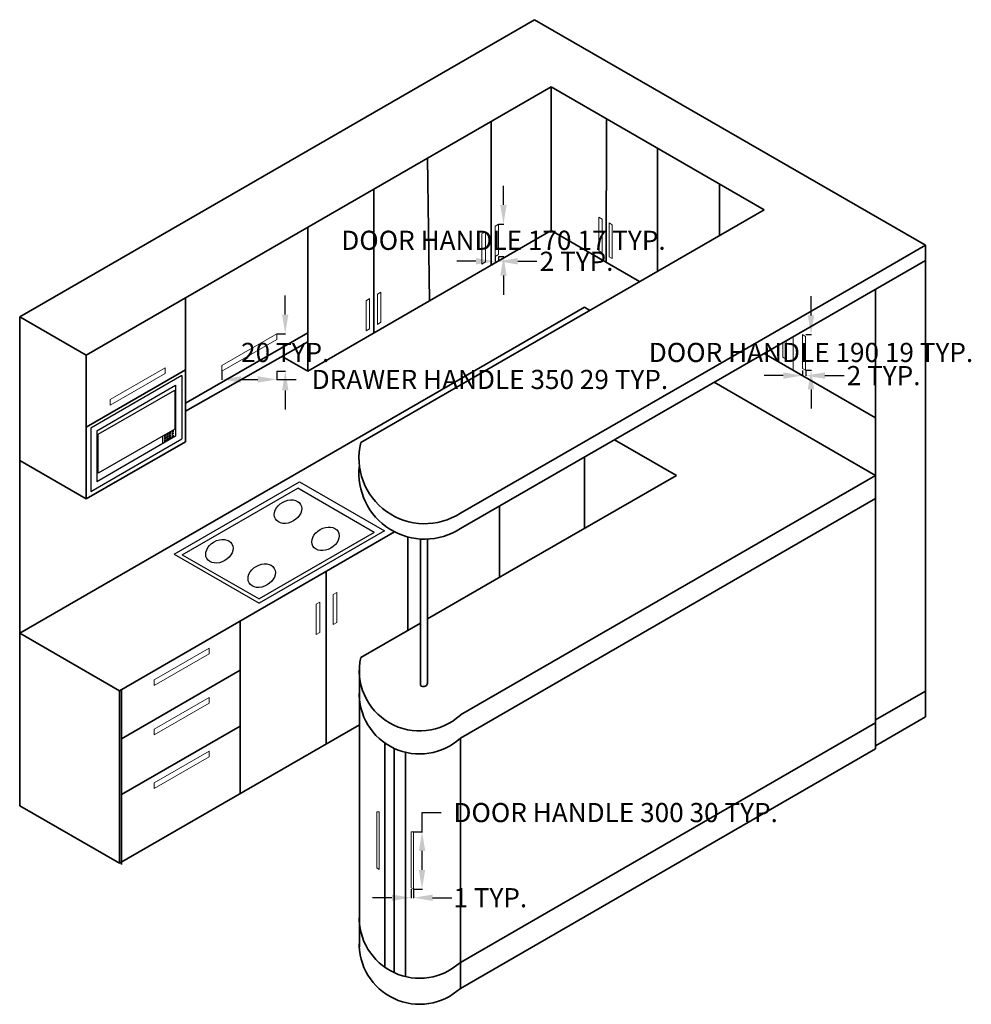
# Model space of a CAD drawing. Units: centimetres. Extents: x 13 to 509, y -97 to 417.
import ezdxf

# ---------------------------------------------------------------- set-up
doc = ezdxf.new("R2010")
doc.units = ezdxf.units.CM
doc.header["$MEASUREMENT"] = 0
for name, color, linetype, lineweight in [('A-ANNO-DIMS', 2, 'Continuous', 18), ('A-EQPM', 4, 'Continuous', 25), ('A-FURN', 7, 'Continuous', 35), ('A-FURN-HDWR', 8, 'Continuous', 18)]:
    doc.layers.add(name, color=color, linetype=linetype, lineweight=lineweight)
doc.styles.get("Standard").update_dxf_attribs({"font": 'arial.ttf'})
doc.dimstyles.get("Standard").update_dxf_attribs({"dimtxt": 10, "dimasz": 10, "dimexe": 0.18, "dimexo": 0.0625, "dimgap": 0.09, "dimtad": 0, "dimtih": 1, "dimtoh": 1, "dimdec": 0, "dimzin": 0, "dimdsep": 46, "dimtxsty": 'Standard', "dimcen": 0.09, "dimadec": 0, "dimazin": 0, "dimtfac": 1, "dimtdec": 0, "dimtofl": 0, "dimtmove": 0, "dimatfit": 3, "dimfxl": 1, "dimtolj": 1, "dimtzin": 0, "dimarcsym": 0})

# ---------------------------------------------------------------- blocks, each defined once
blk = doc.blocks.new('HANDLE-VERT-170')
for p, q in [((0, 15.78), (1.85, 16.85)), ((0, 15.78), (0, 0)), ((1.85, 1.07), (1.85, 16.85)), ((0, 0), (1.85, 1.07))]:
    blk.add_line(p, q)
blk = doc.blocks.new('HANDLE-DIAG-350')
for p, q in [((28.72, 19.54), (0, 2.96)), ((0, 0), (28.72, 16.58)), ((28.72, 16.58), (28.72, 19.54)), ((0, 0), (0, 2.96))]:
    blk.add_line(p, q)
blk = doc.blocks.new('HANDLE-VERT-190')
for p, q in [((1.67, 17.63), (0, 18.59)), ((0, 18.59), (0, 0.97)), ((1.67, 0.02), (1.67, 17.63)), ((1.67, 0), (0, 0.97))]:
    blk.add_line(p, q)
blk = doc.blocks.new('HANDLE-VERT-300')
for p, q in [((0, 0.73), (0, 29.93)), ((1.26, 29.93), (0, 29.93)), ((1.26, 29.93), (1.26, 0)), ((1.26, 0), (0, 0.73))]:
    blk.add_line(p, q)
blk = doc.blocks.new('*D5')
at = {"layer": 'A-ANNO-DIMS', "color": 0, "lineweight": -2, "transparency": 16777216}
for p, q in [((264.84, 320.42), (264.84, 330.42)), ((262.37, 310.42), (265.02, 310.42)), ((262.37, 293.57), (265.02, 293.57)), ((264.84, 283.57), (264.84, 273.57))]:
    blk.add_line(p, q, dxfattribs=at)
at = {"layer": 'A-ANNO-DIMS', "color": 0, "transparency": 16777216}
for points in [[(263.17, 320.42), (266.51, 320.42), (264.84, 310.42)], [(263.17, 283.57), (266.51, 283.57), (264.84, 293.57)]]:
    blk.add_solid(points, dxfattribs=at)
at = {"layer": 'Defpoints', "color": 0, "transparency": 16777216}
for p in [(262.31, 310.42), (264.84, 310.42), (262.31, 293.57)]:
    blk.add_point(p, dxfattribs=at)
at = {"layer": 'A-ANNO-DIMS', "color": 0, "transparency": 16777216, "insert": (264.84, 301.99), "char_height": 10, "attachment_point": 5}
blk.add_mtext('\\A1;DOOR HANDLE 170 17 TYP.', dxfattribs=at)
blk = doc.blocks.new('*D6')
at = {"layer": 'A-ANNO-DIMS', "color": 0, "lineweight": -2, "transparency": 16777216}
for p, q in [((260.46, 293.5), (260.46, 290.86)), ((262.31, 293.5), (262.31, 290.86)), ((250.46, 291.04), (240.46, 291.04)), ((272.31, 291.04), (282.31, 291.04))]:
    blk.add_line(p, q, dxfattribs=at)
at = {"layer": 'A-ANNO-DIMS', "color": 0, "transparency": 16777216}
for points in [[(250.46, 292.71), (250.46, 289.37), (260.46, 291.04)], [(272.31, 292.71), (272.31, 289.37), (262.31, 291.04)]]:
    blk.add_solid(points, dxfattribs=at)
at = {"layer": 'Defpoints', "color": 0, "transparency": 16777216}
for p in [(260.46, 293.57), (262.31, 293.57), (262.31, 291.04)]:
    blk.add_point(p, dxfattribs=at)
at = {"layer": 'A-ANNO-DIMS', "color": 0, "transparency": 16777216, "insert": (302.94, 291.04), "char_height": 10, "attachment_point": 5}
blk.add_mtext('\\A1;2 TYP.', dxfattribs=at)
blk = doc.blocks.new('*D7')
at = {"layer": 'A-ANNO-DIMS', "color": 0, "lineweight": -2, "transparency": 16777216}
for p, q in [((118.02, 233.67), (118.02, 229.24)), ((146.74, 233.67), (146.74, 229.24)), ((128.02, 229.42), (136.74, 229.42)), ((146.74, 229.42), (156.74, 229.42))]:
    blk.add_line(p, q, dxfattribs=at)
at = {"layer": 'A-ANNO-DIMS', "color": 0, "transparency": 16777216}
for points in [[(128.02, 231.09), (128.02, 227.76), (118.02, 229.42)], [(136.74, 231.09), (136.74, 227.76), (146.74, 229.42)]]:
    blk.add_solid(points, dxfattribs=at)
at = {"layer": 'Defpoints', "color": 0, "transparency": 16777216}
for p in [(118.02, 233.73), (146.74, 233.73), (146.74, 229.42)]:
    blk.add_point(p, dxfattribs=at)
at = {"layer": 'A-ANNO-DIMS', "color": 0, "transparency": 16777216, "insert": (257.77, 229.42), "char_height": 10, "attachment_point": 5}
blk.add_mtext('\\A1;DRAWER HANDLE 350 29 TYP.', dxfattribs=at)
blk = doc.blocks.new('*D8')
at = {"layer": 'A-ANNO-DIMS', "color": 0, "lineweight": -2, "transparency": 16777216}
for p, q in [((151.04, 263.28), (151.04, 273.28)), ((146.8, 253.28), (151.22, 253.28)), ((146.8, 233.73), (151.22, 233.73)), ((151.04, 223.73), (151.04, 213.73))]:
    blk.add_line(p, q, dxfattribs=at)
at = {"layer": 'A-ANNO-DIMS', "color": 0, "transparency": 16777216}
for points in [[(149.38, 263.28), (152.71, 263.28), (151.04, 253.28)], [(149.38, 223.73), (152.71, 223.73), (151.04, 233.73)]]:
    blk.add_solid(points, dxfattribs=at)
at = {"layer": 'Defpoints', "color": 0, "transparency": 16777216}
for p in [(146.74, 253.28), (151.04, 253.28), (146.74, 233.73)]:
    blk.add_point(p, dxfattribs=at)
at = {"layer": 'A-ANNO-DIMS', "color": 0, "transparency": 16777216, "insert": (151.04, 243.5), "char_height": 10, "attachment_point": 5}
blk.add_mtext('\\A1;20 TYP.', dxfattribs=at)
blk = doc.blocks.new('*D9')
at = {"layer": 'A-ANNO-DIMS', "color": 0, "lineweight": -2, "transparency": 16777216}
for p, q in [((425.19, 262.8), (425.19, 272.8)), ((422.47, 252.8), (425.37, 252.8)), ((422.47, 234.2), (425.38, 234.21)), ((425.2, 224.21), (425.2, 214.21))]:
    blk.add_line(p, q, dxfattribs=at)
at = {"layer": 'A-ANNO-DIMS', "color": 0, "transparency": 16777216}
for points in [[(426.86, 262.8), (423.52, 262.8), (425.19, 252.8)], [(426.87, 224.21), (423.53, 224.21), (425.2, 234.21)]]:
    blk.add_solid(points, dxfattribs=at)
at = {"layer": 'Defpoints', "color": 0, "transparency": 16777216}
for p in [(422.4, 252.8), (425.19, 252.8), (422.41, 234.2)]:
    blk.add_point(p, dxfattribs=at)
at = {"layer": 'A-ANNO-DIMS', "color": 0, "transparency": 16777216, "insert": (425.19, 243.5), "char_height": 10, "attachment_point": 5}
blk.add_mtext('\\A1;DOOR HANDLE 190 19 TYP.', dxfattribs=at)
blk = doc.blocks.new('*D10')
at = {"layer": 'A-ANNO-DIMS', "color": 0, "lineweight": -2, "transparency": 16777216}
for p, q in [((410.74, 231.41), (400.74, 231.41)), ((420.73, 234.14), (420.74, 231.24)), ((422.41, 234.14), (422.41, 231.24)), ((432.41, 231.42), (442.41, 231.42))]:
    blk.add_line(p, q, dxfattribs=at)
at = {"layer": 'A-ANNO-DIMS', "color": 0, "transparency": 16777216}
for points in [[(410.74, 233.08), (410.74, 229.75), (420.74, 231.42)], [(432.41, 233.08), (432.41, 229.75), (422.41, 231.42)]]:
    blk.add_solid(points, dxfattribs=at)
at = {"layer": 'Defpoints', "color": 0, "transparency": 16777216}
for p in [(420.73, 234.2), (422.41, 234.2), (422.41, 231.42)]:
    blk.add_point(p, dxfattribs=at)
at = {"layer": 'A-ANNO-DIMS', "color": 0, "transparency": 16777216, "insert": (463.04, 231.42), "char_height": 10, "attachment_point": 5}
blk.add_mtext('\\A1;2 TYP.', dxfattribs=at)
blk = doc.blocks.new('*D11')
at = {"layer": 'A-ANNO-DIMS', "color": 0, "lineweight": -2, "transparency": 16777216}
for p, q in [((222.38, -6.5), (222.38, 3.5)), ((222.38, 3.5), (232.38, 3.5)), ((217.95, -6.5), (222.56, -6.5)), ((222.38, -26.43), (222.38, -16.5)), ((217.95, -36.43), (222.56, -36.43))]:
    blk.add_line(p, q, dxfattribs=at)
at = {"layer": 'A-ANNO-DIMS', "color": 0, "transparency": 16777216}
for points in [[(220.71, -16.5), (224.05, -16.5), (222.38, -6.5)], [(220.71, -26.43), (224.05, -26.43), (222.38, -36.43)]]:
    blk.add_solid(points, dxfattribs=at)
at = {"layer": 'Defpoints', "color": 0, "transparency": 16777216}
for p in [(217.89, -6.5), (222.38, -6.5), (217.89, -36.43)]:
    blk.add_point(p, dxfattribs=at)
at = {"layer": 'A-ANNO-DIMS', "color": 0, "transparency": 16777216, "insert": (323.33, 3.5), "char_height": 10, "attachment_point": 5}
blk.add_mtext('\\A1;DOOR HANDLE 300 30 TYP.', dxfattribs=at)
blk = doc.blocks.new('*D12')
at = {"layer": 'A-ANNO-DIMS', "color": 0, "lineweight": -2, "transparency": 16777216}
for p, q in [((206.63, -40.92), (196.63, -40.92)), ((216.63, -36.5), (216.63, -41.1)), ((217.89, -36.5), (217.89, -41.1)), ((227.89, -40.92), (237.89, -40.92))]:
    blk.add_line(p, q, dxfattribs=at)
at = {"layer": 'A-ANNO-DIMS', "color": 0, "transparency": 16777216}
for points in [[(206.63, -39.26), (206.63, -42.59), (216.63, -40.92)], [(227.89, -39.26), (227.89, -42.59), (217.89, -40.92)]]:
    blk.add_solid(points, dxfattribs=at)
at = {"layer": 'Defpoints', "color": 0, "transparency": 16777216}
for p in [(216.63, -36.43), (217.89, -36.43), (217.89, -40.92)]:
    blk.add_point(p, dxfattribs=at)
at = {"layer": 'A-ANNO-DIMS', "color": 0, "transparency": 16777216, "insert": (257.96, -40.92), "char_height": 10, "attachment_point": 5}
blk.add_mtext('\\A1;1 TYP.', dxfattribs=at)

msp = doc.modelspace()

# ---------------------------------------------------------------- linework, layer by layer
at = {"layer": 'A-EQPM'}
for p, q in [((97.19, 231.48), (49.63, 204.02)), ((97.19, 231.48), (97.19, 198.49)), ((52.83, 202.65), (93.87, 226.35)), ((93.87, 226.35), (93.87, 199.77)), ((53.58, 200.81), (93.47, 223.84)), ((93.47, 223.84), (93.47, 203.54)), ((49.63, 204.02), (49.63, 171.03)), ((52.83, 202.65), (52.83, 176.08)), ((93.47, 203.54), (53.58, 180.51)), ((53.58, 180.51), (53.58, 200.81)), ((88.06, 200.06), (88.67, 200.41)), ((88.67, 200.41), (88.67, 199.86)), ((89.27, 200.76), (89.85, 201.1)), ((89.27, 200.76), (89.27, 200.21)), ((89.85, 200.55), (89.27, 200.21)), ((89.85, 201.1), (89.85, 200.55)), ((90.54, 201.49), (91.26, 201.91)), ((90.54, 201.49), (90.54, 200.94)), ((91.27, 201.36), (90.54, 200.94)), ((90.54, 200.34), (91.28, 200.76)), ((90.54, 200.34), (90.54, 199.72)), ((91.26, 201.91), (91.27, 201.36)), ((91.28, 200.76), (91.29, 200.16)), ((92.07, 202.38), (92.68, 202.73)), ((92.07, 202.38), (92.07, 201.82)), ((92.68, 202.17), (92.07, 201.82)), ((92.07, 201.22), (92.68, 201.57)), ((92.07, 201.22), (92.07, 200.61)), ((92.68, 200.96), (92.07, 200.61)), ((92.07, 200.06), (92.68, 200.41)), ((92.68, 202.73), (92.68, 202.17)), ((92.68, 201.57), (92.68, 200.96)), ((92.68, 200.41), (92.68, 199.68)), ((49.63, 171.03), (97.19, 198.49)), ((93.87, 199.77), (52.83, 176.08)), ((87.06, 199.84), (87, 195.8)), ((88.06, 200.06), (88.06, 199.51)), ((88.67, 199.86), (88.06, 199.51)), ((88.06, 198.91), (88.67, 199.26)), ((88.06, 198.91), (88.06, 198.29)), ((88.67, 198.65), (88.06, 198.29)), ((88.06, 197.74), (88.67, 198.09)), ((88.06, 197.74), (88.06, 197.02)), ((88.67, 197.37), (88.06, 197.02)), ((88.67, 199.26), (88.67, 198.65)), ((88.67, 198.09), (88.67, 197.37)), ((89.27, 199.6), (89.85, 199.94)), ((89.27, 199.6), (89.27, 198.99)), ((89.85, 199.33), (89.27, 198.99)), ((89.27, 198.44), (89.85, 198.78)), ((89.27, 198.44), (89.27, 197.71)), ((89.85, 198.05), (89.27, 197.71)), ((89.85, 199.94), (89.85, 199.33)), ((89.85, 198.78), (89.85, 198.05)), ((91.29, 200.16), (90.54, 199.72)), ((90.54, 199.17), (91.3, 199.61)), ((90.54, 199.17), (90.54, 198.45)), ((91.31, 198.9), (90.54, 198.45)), ((91.3, 199.61), (91.31, 198.9)), ((92.07, 200.06), (92.07, 199.33)), ((92.68, 199.68), (92.07, 199.33)), ((93.2, 138.32), (158.53, 176.03)), ((158.53, 176.03), (202.84, 150.45)), ((97.34, 137.87), (157.53, 172.62)), ((197.47, 149.56), (157.53, 172.62)), ((197.47, 149.56), (137.44, 114.9)), ((202.84, 150.45), (137.51, 112.73)), ((93.2, 138.32), (137.51, 112.73)), ((97.34, 137.87), (137.44, 114.9))]:
    msp.add_line(p, q, dxfattribs=at)
for centre in [(152.49, 160.45), (172.04, 146.28), (116.72, 139.8), (138.77, 127.07)]:
    msp.add_ellipse(centre, major_axis=(6.56, 3.79), ratio=0.741283, dxfattribs=at)
at = {"layer": 'A-FURN'}
for p, q in [((255.08, 402.06), (281.06, 417.06)), ((281.06, 417.06), (484.87, 299.39)), ((12.59, 262.06), (255.08, 402.06)), ((47.23, 242.06), (289.72, 382.06)), ((289.72, 307.06), (289.72, 382.06)), ((289.72, 382.06), (400.74, 317.96)), ((318.51, 365.43), (318.45, 290.47)), ((258.48, 364.02), (258.48, 289.02)), ((345.23, 350.01), (345.23, 285.91)), ((226.25, 270.42), (225.29, 344.86)), ((197.3, 253.7), (197.3, 328.7)), ((377.41, 331.43), (377.41, 304.49)), ((400.74, 317.96), (190.42, 196.54)), ((162.79, 308.77), (162.79, 233.77)), ((162.79, 233.77), (289.72, 307.06)), ((289.72, 307.06), (335.78, 280.46)), ((458.89, 284.39), (484.87, 299.39)), ((484.87, 299.39), (484.87, 53.36)), ((242.38, 151.6), (484.87, 291.43)), ((458.89, 284.39), (242.38, 159.64)), ((458.89, 179.39), (458.89, 276.45)), ((98.99, 271.94), (98.99, 196.94)), ((255.08, 237.06), (307.04, 267.06)), ((309.8, 265.46), (307.04, 267.06)), ((12.59, 187.06), (12.59, 262.06)), ((12.59, 262.06), (47.23, 242.06)), ((98.99, 217.07), (162.79, 253.65)), ((98.99, 212.95), (162.79, 248.96)), ((47.23, 242.06), (47.23, 167.06)), ((162.79, 233.77), (149.49, 241.45)), ((400.78, 242.94), (458.89, 209.39)), ((255.08, 237.06), (12.59, 97.06)), ((47.23, 204.56), (98.99, 234.44)), ((458.89, 179.39), (374.78, 227.95)), ((47.23, 167.06), (98.99, 196.94)), ((322.79, 197.97), (354.97, 179.39)), ((12.59, 97.06), (12.59, 187.06)), ((12.59, 187.06), (47.23, 167.06)), ((307.04, 188.88), (307.04, 151.72)), ((242.38, 54.39), (458.89, 179.39)), ((354.97, 179.39), (277.02, 134.39)), ((458.89, 179.39), (458.89, 36.8)), ((242.38, 42.36), (458.89, 167.36)), ((262.77, 163.36), (262.77, 126.16)), ((64.55, 67.06), (208.08, 149.92)), ((215.01, 147.26), (215.01, 98.58)), ((221.55, 69.85), (221.55, 146.2)), ((225.2, 71.74), (225.2, 146.15)), ((277.02, 134.39), (225.2, 104.47)), ((172.44, 129.35), (172.44, 39.35)), ((127.48, 103.39), (127.48, 13.39)), ((221.55, 102.36), (190.42, 84.39)), ((12.59, 7.06), (12.59, 97.06)), ((12.59, 97.06), (64.55, 67.06)), ((127.48, 77.69), (65.71, 42.03)), ((189.69, 78.99), (189.69, -66.56)), ((64.55, 67.06), (64.55, -22.94)), ((65.71, 67.72), (65.71, -23.61)), ((458.89, 51.83), (484.87, 66.83)), ((458.89, 38.36), (484.87, 53.36)), ((64.55, -22.94), (189.69, 49.31)), ((65.71, 12.95), (127.48, 48.62)), ((242.38, -74.62), (458.89, 50.38)), ((242.38, 42.36), (242.38, -88.2)), ((203.02, 39.76), (203.02, -77.22)), ((207.79, -79.98), (207.79, 37)), ((242.38, -88.2), (458.89, 36.8)), ((213.82, 34.9), (213.82, -82.08)), ((12.59, 7.06), (64.55, -22.94))]:
    msp.add_line(p, q, dxfattribs=at)
for centre, radius, start, end in [((223.78, 188.48), 34.32, 166.4215, 302.8186), ((223.78, 180.44), 34.32, 173.2766, 302.8186), ((221.09, 77.51), 31.43, 167.3624, 312.6376), ((221.09, 65.48), 31.43, 177.2966, 312.6376), ((223.11, 71.3), 2.13, 222.8037, 11.9853), ((221.09, -51.5), 31.43, 177.2966, 312.6376), ((221.09, -65.08), 31.43, 167.3624, 167.5233), ((221.09, -65.08), 31.43, 177.2966, 312.6376)]:
    msp.add_arc(centre, radius, start, end, dxfattribs=at)
at = {"layer": 'A-FURN-HDWR'}
for p, q in [((410.58, 248.59), (410.58, 241.03)), ((412.26, 240.09), (412.26, 249.56)), ((415.87, 234.22), (415.87, 251.64)), ((412.26, 240.06), (410.58, 241.03))]:
    msp.add_line(p, q, dxfattribs=at)

# ---------------------------------------------------------------- block references
for name, p in [('HANDLE-VERT-190', (314.64, 295.46)), ('HANDLE-VERT-170', (260.46, 293.57)), ('HANDLE-VERT-170', (253.63, 289.62)), ('HANDLE-VERT-170', (199.12, 258.15)), ('HANDLE-VERT-170', (193.18, 254.72)), ('HANDLE-DIAG-350', (118.02, 233.73)), ('HANDLE-DIAG-350', (59.68, 215.96)), ('HANDLE-VERT-170', (176.12, 101.52)), ('HANDLE-VERT-170', (167.22, 96.38)), ('HANDLE-DIAG-350', (82.62, 69.76)), ('HANDLE-DIAG-350', (82.62, 44)), ('HANDLE-DIAG-350', (82.62, 15.98)), ('HANDLE-VERT-300', (198.76, -26.12)), ('HANDLE-VERT-300', (216.63, -36.43))]:
    msp.add_blockref(name, p, dxfattribs=at)
at = {"layer": 'A-FURN-HDWR', "rotation": 0.0129910890971178}
for p in [(319.87, 292.44), (420.73, 234.2)]:
    msp.add_blockref('HANDLE-VERT-190', p, dxfattribs=at)

# ---------------------------------------------------------------- dimensions: what is measured, and where the dimension line sits
at = {"layer": 'A-ANNO-DIMS'}
for base, p1, p2, angle, text, picture, middle in [((264.84, 310.42), (262.31, 293.57), (262.31, 310.42), 90, 'DOOR HANDLE 170 <> TYP.', '*D5', (264.84, 301.99)), ((425.19, 252.8), (422.41, 234.2), (422.4, 252.8), 90.013, 'DOOR HANDLE 190 <> TYP.', '*D9', (425.19, 243.5)), ((151.04, 253.28), (146.74, 233.73), (146.74, 253.28), 90, '<> TYP.', '*D8', (151.04, 243.5)), ((422.41, 231.42), (420.73, 234.2), (422.41, 234.2), 0.013, '<> TYP.', '*D10', (463.04, 231.42)), ((222.38, -6.5), (217.89, -36.43), (217.89, -6.5), 90, 'DOOR HANDLE 300 <> TYP.', '*D11', (323.33, 3.5))]:
    dim = msp.add_linear_dim(base=base, p1=p1, p2=p2, angle=angle, text=text, dimstyle='Standard', override={"dimdec": 0, "dimlfac": 1, "dimrnd": 0, "dimzin": 0, "dimdsep": 46, "dimlunit": 2}, dxfattribs=at)
    dim.commit()
    dim.dimension.update_dxf_attribs({"geometry": picture, "text_midpoint": middle})
for base, p1, p2, text, picture, middle in [((262.31, 291.04), (260.46, 293.57), (262.31, 293.57), '<> TYP.', '*D6', (302.94, 291.04)), ((146.74, 229.42), (118.02, 233.73), (146.74, 233.73), 'DRAWER HANDLE 350 <> TYP.', '*D7', (257.77, 229.42)), ((217.89, -40.92), (216.63, -36.43), (217.89, -36.43), '<> TYP.', '*D12', (257.96, -40.92))]:
    dim = msp.add_linear_dim(base=base, p1=p1, p2=p2, text=text, dimstyle='Standard', override={"dimdec": 0, "dimlfac": 1, "dimrnd": 0, "dimzin": 0, "dimdsep": 46, "dimlunit": 2}, dxfattribs=at)
    dim.commit()
    dim.dimension.update_dxf_attribs({"geometry": picture, "text_midpoint": middle})

doc.saveas('drawing.dxf')
